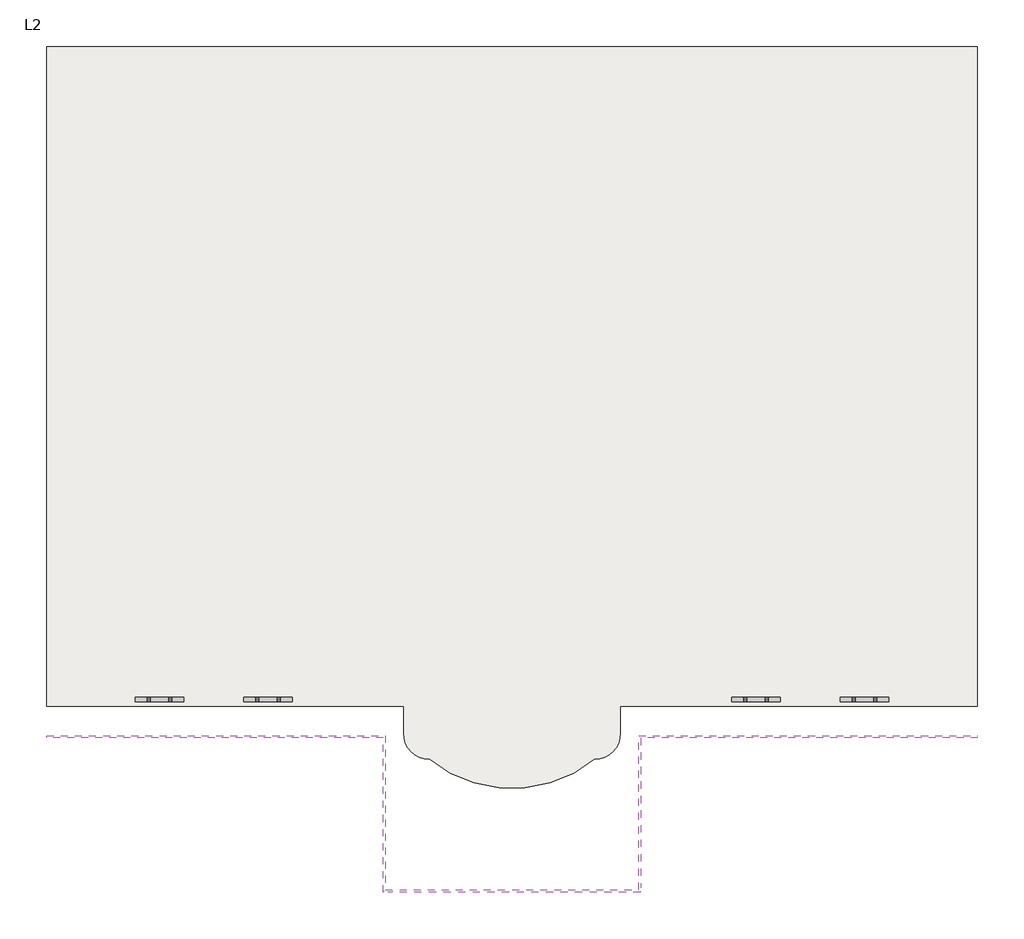
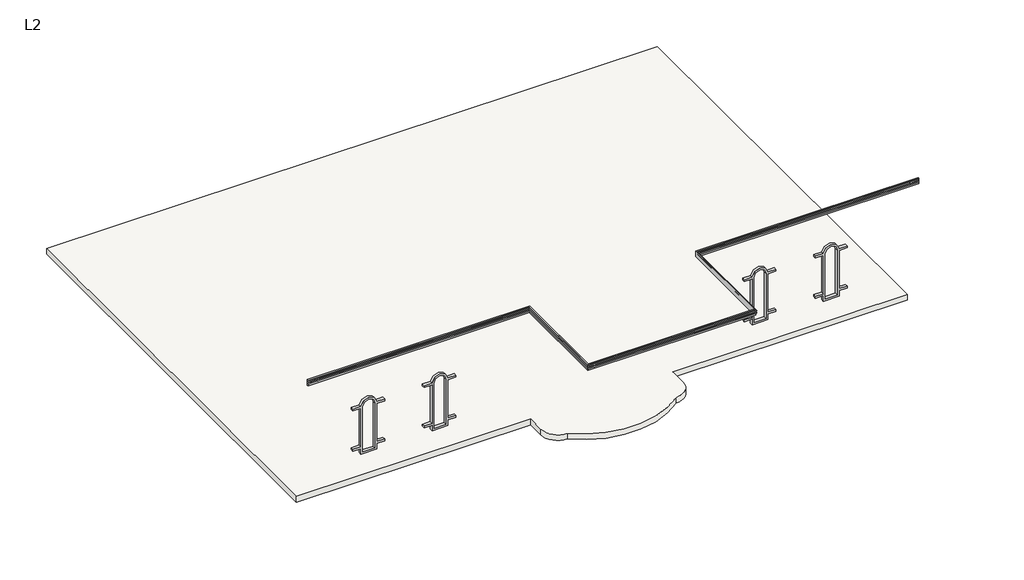
# One storey, incomplete: 5 proxies, 1 slab.
"""IFC4 building model written with IfcOpenShell, lengths in millimetres."""

from ifc_helpers import new_model, si_unit, point, frame, frame_2d, origin, place, context, project, spatial, polyline, circle_curve, trimmed, segment, composite_curve, outline, extrude, transform, mapped, element, save
from components import generic_models_1_generic_models_1_e4eb0336, generic_models_19_generic_models_19_d22e943b

model = new_model("IFC4")

# Units and contexts
model_context = context("Model", 3, world=origin())
ifc_project = project(units=[si_unit("LENGTHUNIT", "METRE", prefix="MILLI")], contexts=[model_context])

# Site, building, storey
site = spatial("IfcSite", under=ifc_project)
building = spatial("IfcBuilding", under=site)
storey = spatial("IfcBuildingStorey", under=building, Name="L2", Elevation=3048.0)

# Proxies
placement = place(None, origin())
generic_models_1_generic_models_1_shape = generic_models_1_generic_models_1_e4eb0336(model_context)
element("IfcBuildingElementProxy", 1, Name="Generic Models 1 : Generic Models 1", ObjectType="Generic Models 1 : Generic Models 1", at=placement, inside=storey, context=model_context, shape_type="MappedRepresentation", body=[
    mapped(generic_models_1_generic_models_1_shape, transform((0.0, 0.0, 0.0), x_axis=(1.0, 0.0, 0.0), y_axis=(0.0, 1.0, 0.0), z_axis=(0.0, 0.0, 1.0))),
])
generic_models_19_generic_models_19_shape = generic_models_19_generic_models_19_d22e943b(model_context)
element("IfcBuildingElementProxy", 2, Name="Generic Models 19 : Generic Models 19", ObjectType="Generic Models 19 : Generic Models 19", at=placement, inside=storey, context=model_context, shape_type="MappedRepresentation", body=[
    mapped(generic_models_19_generic_models_19_shape, transform((0.0, 0.0, 0.0), x_axis=(1.0, 0.0, 0.0), y_axis=(0.0, 1.0, 0.0), z_axis=(0.0, 0.0, 1.0))),
])
element("IfcBuildingElementProxy", 3, Name="Generic Models 2 : Generic Models 1", ObjectType="Generic Models 2 : Generic Models 1", at=placement, inside=storey, context=model_context, shape_type="MappedRepresentation", body=[
    mapped(generic_models_1_generic_models_1_shape, transform((1828.8, 0.0, 0.0), x_axis=(1.0, 0.0, 0.0), y_axis=(0.0, 1.0, 0.0), z_axis=(0.0, 0.0, 1.0))),
])
element("IfcBuildingElementProxy", 4, Name="Generic Models 3 : Generic Models 1", ObjectType="Generic Models 3 : Generic Models 1", at=placement, inside=storey, context=model_context, shape_type="MappedRepresentation", body=[
    mapped(generic_models_1_generic_models_1_shape, transform((10058.4, 0.0, 0.0), x_axis=(1.0, 0.0, 0.0), y_axis=(0.0, 1.0, 0.0), z_axis=(0.0, 0.0, 1.0))),
])
element("IfcBuildingElementProxy", 5, Name="Generic Models 4 : Generic Models 1", ObjectType="Generic Models 4 : Generic Models 1", at=placement, inside=storey, context=model_context, shape_type="MappedRepresentation", body=[
    mapped(generic_models_1_generic_models_1_shape, transform((11887.2, 0.0, 0.0), x_axis=(1.0, 0.0, 0.0), y_axis=(0.0, 1.0, 0.0), z_axis=(0.0, 0.0, 1.0))),
])

# Slab
element("IfcSlab", 6, ObjectType="6\"", at=placement, inside=storey, context=model_context, shape_type="SweptSolid", body=[
    extrude(outline(composite_curve([segment(polyline([(6935.9174924, 6238.7391705), (6935.9174924, -4886.4608295), (916.1174924, -4886.4608295), (916.1174924, -5343.6608295)]), True, "CONTINUOUS"), segment(trimmed(circle_curve(frame_2d((485.0651986, -5343.6608295)), 431.0522938), [point((916.1174924, -5343.6608295))], [point((485.0651986, -5774.7131233))], False, "CARTESIAN"), True, "CONTINUOUS"), segment(trimmed(circle_curve(frame_2d((-912.6825076, -4051.5042958)), 2218.816647), [point((485.0651986, -5774.7131233))], [point((-2310.4302138, -5774.7131233))], False, "CARTESIAN"), True, "CONTINUOUS"), segment(trimmed(circle_curve(frame_2d((-2310.4302138, -5343.6608295)), 431.0522938), [point((-2310.4302138, -5774.7131233))], [point((-2741.4825076, -5343.6608295))], False, "CARTESIAN"), True, "CONTINUOUS"), segment(polyline([(-2741.4825076, -5343.6608295), (-2741.4825076, -4886.4608295), (-8761.2825076, -4886.4608295), (-8761.2825076, 6238.7391705), (6935.9174924, 6238.7391705)]), True, "CONTINUOUS")], self_intersect=False)), frame((0.0, 0.0, 2895.6), z_axis=(0.0, 0.0, 1.0), x_axis=(1.0, 0.0, 0.0)), (0.0, 0.0, 1.0), 152.4),
])

save(model, "model.ifc")

# Revit data of these elements
# Type "6\""
#   Description = "Generic Floor (Material By Category), 12\" thick"
#   Assembly Code = "B1010"
#   Type Mark = "G01"
#   Function = 0
#   Layers, outside or top first: 0' - 6" no material (function 1)
# Element 1 (IfcBuildingElementProxy, "Generic Models 1 : Generic Models 1")
#   Phase Created = New Construction
#   Materials on its faces: "Aluminum"
# Element 2 (IfcBuildingElementProxy, "Generic Models 19 : Generic Models 19")
#   Phase Created = New Construction
# Element 3 (IfcBuildingElementProxy, "Generic Models 2 : Generic Models 1")
#   Phase Created = New Construction
#   Materials on its faces: "Aluminum"
# Element 4 (IfcBuildingElementProxy, "Generic Models 3 : Generic Models 1")
#   Phase Created = New Construction
#   Materials on its faces: "Aluminum"
# Element 5 (IfcBuildingElementProxy, "Generic Models 4 : Generic Models 1")
#   Phase Created = New Construction
#   Materials on its faces: "Aluminum"
# Element 6 (IfcSlab, "6\"")
#   Height Offset From Level = 0' - 0"
#   Phase Created = New Construction
#   Materials on its faces: "Default Floor"
# Materials
#   "Aluminum": class "Metal", colour RGB 244 245 246, transparency 0, Description = "Aluminum 6061", Cost = 0
#   "Default Floor": colour RGB 128 128 128, transparency 0, Cost = 0
